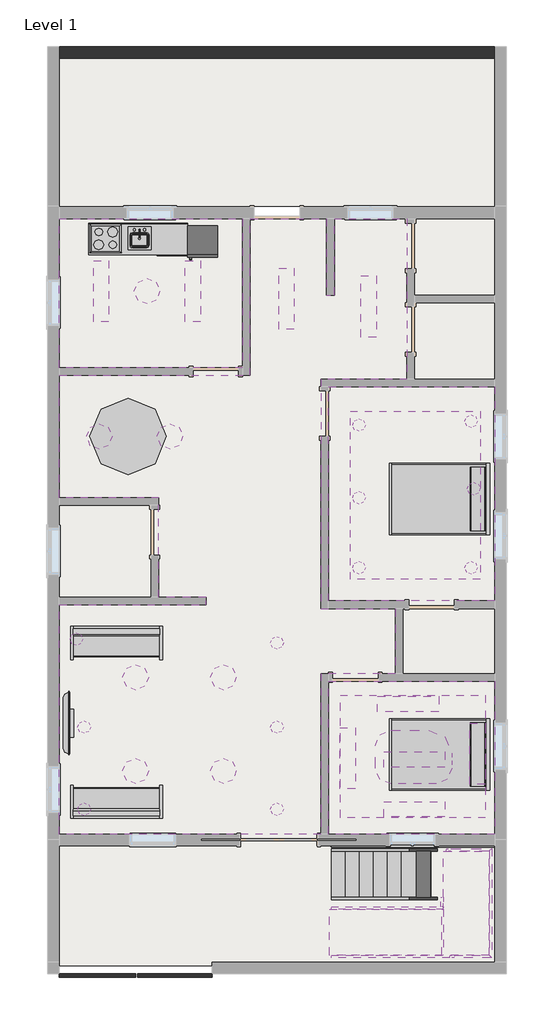
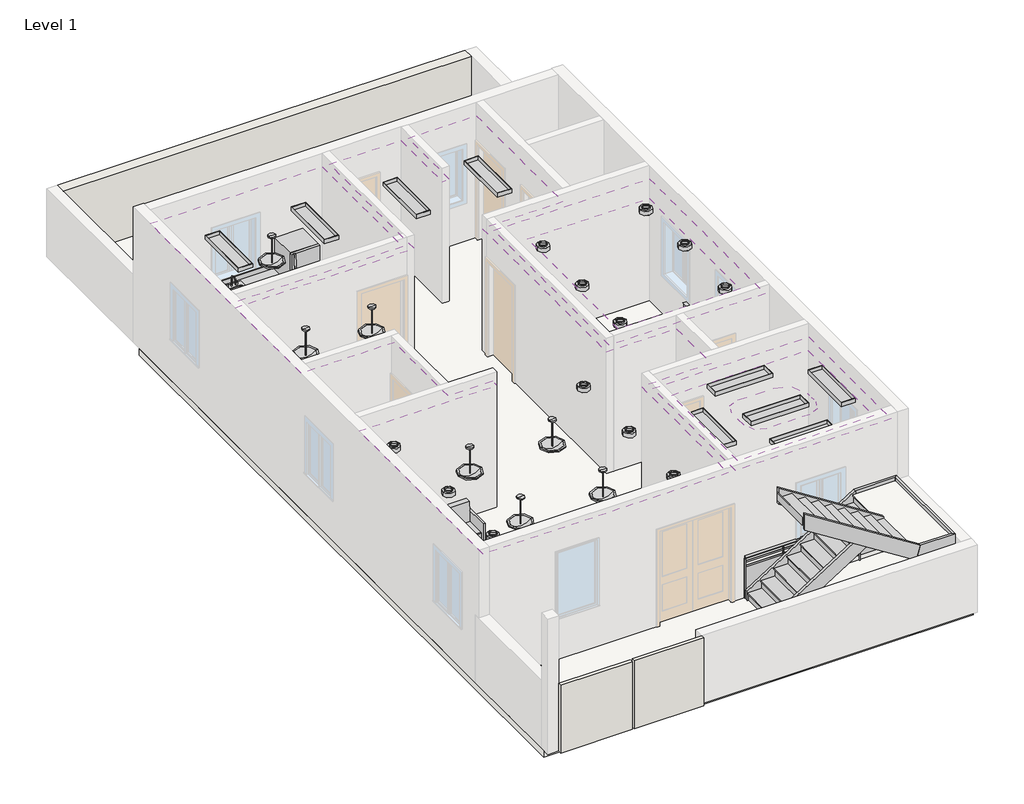
# One storey, part 2 of 2: 28 light fixtures, 8 members, 7 coverings, 7 furniture elements, 4 proxies, 3 slabs, 2 stair flights, 2 walls, 2 other elements.
"""IFC4 building model written with IfcOpenShell, lengths in millimetres."""

from ifc_helpers import new_model, si_unit, point, frame, frame_2d, origin, origin_with_axes, place, context, project, spatial, polyline, circle_curve, ellipse_curve, trimmed, segment, composite_curve, outline, extrude, faceted_brep, transform, mapped, element, save
from ifc_brep_helpers import plane_surface, extruded_surface, advanced_brep
from components import proxy_a6faaae8, proxy_45b28599, kitchenette_medium_kitchenette_medium_844211aa, proxy_c523a7b7, flow_terminal_871c2e40, furniture_096e7f55, furniture_c6510c7c, m_sofa_1830mm_f9e8a66b, furniture_fdf74506, furniture_bbcc68ce, ceiling_light_flat_round_60w_120v_0a96185f, ceiling_light_linear_box_1_x4_1_lamp_120v_8873ebfc, pendant_light_hemisphere_100w_120v_9c66a66f, non_monolithic_landing_9c4d403a, stair_flight_350f2e97, stair_flight_9d7122d5, walls_1_walls_1_5f19503e

model = new_model("IFC4")

# Units and contexts
model_context = context("Model", 3, world=origin())
ifc_project = project(units=[si_unit("LENGTHUNIT", "METRE", prefix="MILLI")], contexts=[model_context])

# Site, building, storey
site = spatial("IfcSite", under=ifc_project)
building = spatial("IfcBuilding", under=site)
storey = spatial("IfcBuildingStorey", under=building, Name="Level 1", Elevation=0.0)

# Proxies
placement = place(None, origin())
proxy_shape = proxy_a6faaae8(model_context)
element("IfcBuildingElementProxy", 1, Name="Cook Top-4 Unit2 : 22\" x 20\"", ObjectType="Cook Top-4 Unit2 : 22\" x 20\"", at=placement, inside=storey, context=model_context, shape_type="MappedRepresentation", body=[
    mapped(proxy_shape, transform((-8913.4692849, 13575.3206867, 0.0), x_axis=(1.0, 0.0, 0.0), y_axis=(0.0, 1.0, 0.0), z_axis=(0.0, 0.0, 1.0))),
])
proxy_2_shape = proxy_45b28599(model_context)
element("IfcBuildingElementProxy", 2, Name="Dishwasher : 24\" x 24\" x 34\"", ObjectType="Dishwasher : 24\" x 24\" x 34\"", at=placement, inside=storey, context=model_context, shape_type="MappedRepresentation", body=[
    mapped(proxy_2_shape, transform((-7962.2867534, 13283.4711219, 0.0), x_axis=(1.0, 0.0, 0.0), y_axis=(0.0, 1.0, 0.0), z_axis=(0.0, 0.0, 1.0))),
])
kitchenette_medium_kitchenette_medium_shape = kitchenette_medium_kitchenette_medium_844211aa(model_context)
element("IfcBuildingElementProxy", 3, Name="Kitchenette - Medium : Kitchenette - Medium", ObjectType="Kitchenette - Medium : Kitchenette - Medium", at=placement, inside=storey, context=model_context, shape_type="MappedRepresentation", body=[
    mapped(kitchenette_medium_kitchenette_medium_shape, transform((-8589.3069898, 13880.1206867, 0.0), x_axis=(1.0, 0.0, 0.0), y_axis=(0.0, 1.0, 0.0), z_axis=(0.0, 0.0, 1.0))),
])
proxy_3_shape = proxy_c523a7b7(model_context)
element("IfcBuildingElementProxy", 4, Name="Refrigerator : 24\" x 25\" LH", ObjectType="Refrigerator : 24\" x 25\" LH", at=placement, inside=storey, context=model_context, shape_type="MappedRepresentation", body=[
    mapped(proxy_3_shape, transform((-6976.7192849, 13529.6717152, 0.0), x_axis=(1.0, 0.0, 0.0), y_axis=(0.0, 1.0, 0.0), z_axis=(0.0, 0.0, 1.0))),
])

# Coverings
element("IfcCovering", 5, ObjectType="2' x 4' ACT System", at=placement, inside=storey, context=model_context, shape_type="SweptSolid", body=[
    extrude(outline(polyline([(-1153.7692849, 6349.0206867), (-4468.4692849, 6349.0206867), (-4468.4692849, 10616.2206867), (-1153.7692849, 10616.2206867), (-1153.7692849, 6349.0206867)])), frame((0.0, 0.0, 2743.2), z_axis=(0.0, 0.0, 1.0), x_axis=(1.0, 0.0, 0.0)), (0.0, 0.0, 1.0), 57.15),
])
element("IfcCovering", 6, ObjectType="2' x 4' ACT System", at=placement, inside=storey, context=model_context, shape_type="SweptSolid", body=[
    extrude(outline(polyline([(-1153.7692849, 1700.8206867), (-4468.4692849, 1700.8206867), (-4468.4692849, 4748.8206867), (-1153.7692849, 4748.8206867), (-1153.7692849, 1700.8206867)])), frame((0.0, 0.0, 2743.2), z_axis=(0.0, 0.0, 1.0), x_axis=(1.0, 0.0, 0.0)), (0.0, 0.0, 1.0), 57.15),
])
element("IfcCovering", 7, ObjectType="2' x 4' ACT System", at=placement, inside=storey, context=model_context, shape_type="SweptSolid", body=[
    extrude(outline(polyline([(-4620.8692849, 4901.2206867), (-4620.8692849, 1700.8206867), (-9840.5692849, 1700.8206867), (-9840.5692849, 6272.8206867), (-6906.8692849, 6272.8206867), (-6906.8692849, 6425.2206867), (-7859.3692849, 6425.2206867), (-7859.3692849, 8406.4206867), (-9840.5692849, 8406.4206867), (-9840.5692849, 10844.8206867), (-6030.5692849, 10844.8206867), (-6030.5692849, 13969.0206867), (-4506.5692849, 13969.0206867), (-4506.5692849, 12445.0206867), (-4354.1692849, 12445.0206867), (-4354.1692849, 13969.0206867), (-2906.3692849, 13969.0206867), (-2906.3692849, 10768.6206867), (-4620.8692849, 10768.6206867), (-4620.8692849, 6196.6206867), (-3134.9692849, 6196.6206867), (-3134.9692849, 4901.2206867), (-4620.8692849, 4901.2206867)])), frame((0.0, 0.0, 2743.2), z_axis=(0.0, 0.0, 1.0), x_axis=(1.0, 0.0, 0.0)), (0.0, 0.0, 1.0), 57.15),
])
element("IfcCovering", 8, ObjectType="2' x 4' ACT System", at=placement, inside=storey, context=model_context, shape_type="SweptSolid", body=[
    extrude(outline(polyline([(-9840.5692849, 13969.0206867), (-6182.9692849, 13969.0206867), (-6182.9692849, 10997.2206867), (-9840.5692849, 10997.2206867), (-9840.5692849, 13969.0206867)])), frame((0.0, 0.0, 2743.2), z_axis=(0.0, 0.0, 1.0), x_axis=(1.0, 0.0, 0.0)), (0.0, 0.0, 1.0), 57.15),
])
element("IfcCovering", 9, ObjectType="design", at=placement, inside=storey, context=model_context, shape_type="SweptSolid", body=[
    extrude(outline(polyline([(-1440.6811411, 10131.5450067), (-1440.6811411, 6778.7450067), (-4031.4811411, 6778.7450067), (-4031.4811411, 10131.5450067), (-1440.6811411, 10131.5450067)]), holes=[composite_curve([segment(polyline([(-1960.6193665, 9832.8150154), (-3523.4811411, 9832.8150154)]), True, "CONTINUOUS"), segment(trimmed(circle_curve(frame_2d((-3523.4811411, 9629.6150154)), 203.2), [point((-3523.4811411, 9832.8150154))], [point((-3726.6811411, 9629.6150154))], True, "CARTESIAN"), True, "CONTINUOUS"), segment(polyline([(-3726.6811411, 9629.6150154), (-3726.6811411, 7369.0150154)]), True, "CONTINUOUS"), segment(trimmed(circle_curve(frame_2d((-3396.4811411, 7369.0150154)), 330.2), [point((-3726.6811411, 7369.0150154))], [point((-3396.4811411, 7038.8150154))], True, "CARTESIAN"), True, "CONTINUOUS"), segment(polyline([(-3396.4811411, 7038.8150154), (-2177.2811411, 7038.8150154)]), True, "CONTINUOUS"), segment(trimmed(circle_curve(frame_2d((-2177.2811411, 7470.6150154)), 431.8), [point((-2177.2811411, 7038.8150154))], [point((-1745.4811411, 7470.6150154))], True, "CARTESIAN"), True, "CONTINUOUS"), segment(polyline([(-1745.4811411, 7470.6150154), (-1745.4811411, 9617.67679)]), True, "CONTINUOUS"), segment(trimmed(circle_curve(frame_2d((-1960.6193665, 9617.67679)), 215.1382254), [point((-1745.4811411, 9617.67679))], [point((-1960.6193665, 9832.8150154))], True, "CARTESIAN"), True, "CONTINUOUS")], self_intersect=False)]), frame((0.0, 0.0, 2692.4), z_axis=(0.0, 0.0, 1.0), x_axis=(1.0, 0.0, 0.0)), (0.0, 0.0, 1.0), 50.8),
])
element("IfcCovering", 10, ObjectType="design", at=placement, inside=storey, context=model_context, shape_type="SweptSolid", body=[
    extrude(outline(polyline([(-1336.3091854, 4467.6615302), (-1336.3091854, 2029.2615302), (-4231.9091854, 2029.2615302), (-4231.9091854, 4467.6615302), (-1336.3091854, 4467.6615302)]), holes=[polyline([(-1663.6359703, 4145.0635701), (-3949.6359703, 4145.0635701), (-3949.6359703, 2316.2635701), (-1663.6359703, 2316.2635701), (-1663.6359703, 4145.0635701)])]), frame((0.0, 0.0, 2679.6205268), z_axis=(0.0, 0.0, 1.0), x_axis=(1.0, 0.0, 0.0)), (0.0, 0.0, 1.0), 50.8),
])
element("IfcCovering", 11, ObjectType="inner", at=placement, inside=storey, context=model_context, shape_type="SweptSolid", body=[
    extrude(outline(composite_curve([segment(trimmed(circle_curve(frame_2d((-2466.1469386, 3312.9178401)), 457.2), [point((-2466.1469386, 3770.1178401))], [point((-2008.9469386, 3312.9178401))], False, "CARTESIAN"), True, "CONTINUOUS"), segment(polyline([(-2008.9469386, 3312.9178401), (-2008.9469386, 3008.1178401)]), True, "CONTINUOUS"), segment(trimmed(circle_curve(frame_2d((-2313.7469386, 3008.1178401)), 304.8), [point((-2008.9469386, 3008.1178401))], [point((-2313.7469386, 2703.3178401))], False, "CARTESIAN"), True, "CONTINUOUS"), segment(polyline([(-2313.7469386, 2703.3178401), (-3228.1469386, 2703.3178401)]), True, "CONTINUOUS"), segment(trimmed(circle_curve(frame_2d((-3228.1469386, 3008.1178401)), 304.8), [point((-3228.1469386, 2703.3178401))], [point((-3532.9469386, 3008.1178401))], False, "CARTESIAN"), True, "CONTINUOUS"), segment(polyline([(-3532.9469386, 3008.1178401), (-3532.9469386, 3465.3178401)]), True, "CONTINUOUS"), segment(trimmed(circle_curve(frame_2d((-3228.1469386, 3465.3178401)), 304.8), [point((-3532.9469386, 3465.3178401))], [point((-3228.1469386, 3770.1178401))], False, "CARTESIAN"), True, "CONTINUOUS"), segment(polyline([(-3228.1469386, 3770.1178401), (-2466.1469386, 3770.1178401)]), True, "CONTINUOUS")], self_intersect=False)), frame((0.0, 0.0, 2641.6), z_axis=(0.0, 0.0, 1.0), x_axis=(1.0, 0.0, 0.0)), (0.0, 0.0, 1.0), 50.8),
])

# Flow terminal
flow_terminal_shape = flow_terminal_871c2e40(model_context)
element("IfcFlowTerminal", 12, ObjectType="Sink Kitchen-Island : 18\" x 18\"", at=placement, inside=storey, context=model_context, shape_type="MappedRepresentation", body=[
    mapped(flow_terminal_shape, transform((-8256.0585254, 13572.9752855, -14.4), x_axis=(1.0, 0.0, 0.0), y_axis=(0.0, 1.0, 0.0), z_axis=(0.0, 0.0, 1.0))),
])

# Furniture
furniture_shape = furniture_096e7f55(model_context)
element("IfcFurniture", 13, ObjectType="Bed-Shaker : Double 56\" x 78\"", at=placement, inside=storey, context=model_context, shape_type="MappedRepresentation", body=[
    mapped(furniture_shape, transform((-1268.0692849, 8361.9706867, 0.0), x_axis=(0.0, -1.0000000000000007, 0.0), y_axis=(1.0000000000000007, 0.0, 0.0), z_axis=(0.0, 0.0, 1.0))),
])
element("IfcFurniture", 14, ObjectType="Bed-Shaker : Double 56\" x 78\"", at=placement, inside=storey, context=model_context, shape_type="MappedRepresentation", body=[
    mapped(furniture_shape, transform((-1268.0692849, 3269.2706867, 0.0), x_axis=(0.0, -1.0, 0.0), y_axis=(1.0, 0.0, 0.0), z_axis=(0.0, 0.0, 1.0))),
])
furniture_2_shape = furniture_c6510c7c(model_context)
element("IfcFurniture", 15, ObjectType="Counter Top w Sink Hole : 24\" Depth", at=placement, inside=storey, context=model_context, shape_type="MappedRepresentation", body=[
    mapped(furniture_2_shape, transform((-8055.9069898, 13880.1206867, -14.4), x_axis=(1.0, 0.0, 0.0), y_axis=(0.0, 1.0, 0.0), z_axis=(0.0, 0.0, 1.0))),
])
m_sofa_1830mm_shape = m_sofa_1830mm_f9e8a66b(model_context)
element("IfcFurniture", 16, ObjectType="M_Sofa : 1830mm", at=placement, inside=storey, context=model_context, shape_type="MappedRepresentation", body=[
    mapped(m_sofa_1830mm_shape, transform((-8767.9397767, 5364.6665883, 0.0), x_axis=(1.0, 0.0, 0.0), y_axis=(0.0, 1.0, 0.0), z_axis=(0.0, 0.0, 1.0))),
])
element("IfcFurniture", 17, ObjectType="M_Sofa : 1830mm", at=placement, inside=storey, context=model_context, shape_type="MappedRepresentation", body=[
    mapped(m_sofa_1830mm_shape, transform((-8627.1987931, 2494.674785, 0.0), x_axis=(-1.0000000000000002, 0.0, 0.0), y_axis=(0.0, -1.0000000000000002, 0.0), z_axis=(0.0, 0.0, 1.0))),
])
furniture_3_shape = furniture_fdf74506(model_context)
element("IfcFurniture", 18, ObjectType="TV - Flat Screen : 50\"", at=placement, inside=storey, context=model_context, shape_type="MappedRepresentation", body=[
    mapped(furniture_3_shape, transform((-9706.3630954, 3915.2652008, 0.0), x_axis=(0.0, 1.0000000000000007, 0.0), y_axis=(-1.0000000000000007, 0.0, 0.0), z_axis=(0.0, 0.0, 1.0))),
])
furniture_4_shape = furniture_bbcc68ce(model_context)
element("IfcFurniture", 19, ObjectType="Table-Dining Round w Chairs : 60\" Diameter", at=placement, inside=storey, context=model_context, shape_type="MappedRepresentation", body=[
    mapped(furniture_4_shape, transform((-8572.6512521, 9810.4993752, 0.0), x_axis=(1.0, 0.0, 0.0), y_axis=(0.0, 1.0, 0.0), z_axis=(0.0, 0.0, 1.0))),
])

# Light fixtures
ceiling_light_flat_round_60w_120v_shape = ceiling_light_flat_round_60w_120v_0a96185f(model_context)
element("IfcLightFixture", 20, ObjectType="Ceiling Light - Flat Round : 60W - 120V", at=placement, inside=storey, context=model_context, shape_type="MappedRepresentation", body=[
    mapped(ceiling_light_flat_round_60w_120v_shape, transform((-9497.6692849, 5587.0206867, 304.8), x_axis=(1.0, 0.0, 0.0), y_axis=(0.0, 1.0, 0.0), z_axis=(0.0, 0.0, 1.0))),
])
element("IfcLightFixture", 21, ObjectType="Ceiling Light - Flat Round : 60W - 120V", at=placement, inside=storey, context=model_context, shape_type="MappedRepresentation", body=[
    mapped(ceiling_light_flat_round_60w_120v_shape, transform((-5497.1692849, 5510.8206867, 304.8), x_axis=(1.0, 0.0, 0.0), y_axis=(0.0, 1.0, 0.0), z_axis=(0.0, 0.0, 1.0))),
])
element("IfcLightFixture", 22, ObjectType="Ceiling Light - Flat Round : 60W - 120V", at=placement, inside=storey, context=model_context, shape_type="MappedRepresentation", body=[
    mapped(ceiling_light_flat_round_60w_120v_shape, transform((-9345.2692849, 3834.4206867, 304.8), x_axis=(1.0, 0.0, 0.0), y_axis=(0.0, 1.0, 0.0), z_axis=(0.0, 0.0, 1.0))),
])
element("IfcLightFixture", 23, ObjectType="Ceiling Light - Flat Round : 60W - 120V", at=placement, inside=storey, context=model_context, shape_type="MappedRepresentation", body=[
    mapped(ceiling_light_flat_round_60w_120v_shape, transform((-5497.1692849, 3834.4206867, 304.8), x_axis=(1.0, 0.0, 0.0), y_axis=(0.0, 1.0, 0.0), z_axis=(0.0, 0.0, 1.0))),
])
element("IfcLightFixture", 24, ObjectType="Ceiling Light - Flat Round : 60W - 120V", at=placement, inside=storey, context=model_context, shape_type="MappedRepresentation", body=[
    mapped(ceiling_light_flat_round_60w_120v_shape, transform((-9345.2692849, 2196.1206867, 304.8), x_axis=(1.0, 0.0, 0.0), y_axis=(0.0, 1.0, 0.0), z_axis=(0.0, 0.0, 1.0))),
])
element("IfcLightFixture", 25, ObjectType="Ceiling Light - Flat Round : 60W - 120V", at=placement, inside=storey, context=model_context, shape_type="MappedRepresentation", body=[
    mapped(ceiling_light_flat_round_60w_120v_shape, transform((-5497.1692849, 2196.1206867, 304.8), x_axis=(1.0, 0.0, 0.0), y_axis=(0.0, 1.0, 0.0), z_axis=(0.0, 0.0, 1.0))),
])
element("IfcLightFixture", 26, ObjectType="Ceiling Light - Flat Round : 60W - 277V", at=placement, inside=storey, context=model_context, shape_type="MappedRepresentation", body=[
    mapped(ceiling_light_flat_round_60w_120v_shape, transform((-3858.8692849, 9854.2206867, 254.0), x_axis=(1.0, 0.0, 0.0), y_axis=(0.0, 1.0, 0.0), z_axis=(0.0, 0.0, 1.0))),
])
element("IfcLightFixture", 27, ObjectType="Ceiling Light - Flat Round : 60W - 277V", at=placement, inside=storey, context=model_context, shape_type="MappedRepresentation", body=[
    mapped(ceiling_light_flat_round_60w_120v_shape, transform((-1623.6692849, 9930.4206867, 254.0), x_axis=(1.0, 0.0, 0.0), y_axis=(0.0, 1.0, 0.0), z_axis=(0.0, 0.0, 1.0))),
])
element("IfcLightFixture", 28, ObjectType="Ceiling Light - Flat Round : 60W - 277V", at=placement, inside=storey, context=model_context, shape_type="MappedRepresentation", body=[
    mapped(ceiling_light_flat_round_60w_120v_shape, transform((-1572.8692849, 8584.2206867, 254.0), x_axis=(1.0, 0.0, 0.0), y_axis=(0.0, 1.0, 0.0), z_axis=(0.0, 0.0, 1.0))),
])
element("IfcLightFixture", 29, ObjectType="Ceiling Light - Flat Round : 60W - 277V", at=placement, inside=storey, context=model_context, shape_type="MappedRepresentation", body=[
    mapped(ceiling_light_flat_round_60w_120v_shape, transform((-3858.8692849, 8406.4206867, 254.0), x_axis=(1.0, 0.0, 0.0), y_axis=(0.0, 1.0, 0.0), z_axis=(0.0, 0.0, 1.0))),
])
element("IfcLightFixture", 30, ObjectType="Ceiling Light - Flat Round : 60W - 277V", at=placement, inside=storey, context=model_context, shape_type="MappedRepresentation", body=[
    mapped(ceiling_light_flat_round_60w_120v_shape, transform((-3858.8692849, 7009.4206867, 254.0), x_axis=(1.0, 0.0, 0.0), y_axis=(0.0, 1.0, 0.0), z_axis=(0.0, 0.0, 1.0))),
])
element("IfcLightFixture", 31, ObjectType="Ceiling Light - Flat Round : 60W - 277V", at=placement, inside=storey, context=model_context, shape_type="MappedRepresentation", body=[
    mapped(ceiling_light_flat_round_60w_120v_shape, transform((-1623.6692849, 7009.4206867, 254.0), x_axis=(1.0, 0.0, 0.0), y_axis=(0.0, 1.0, 0.0), z_axis=(0.0, 0.0, 1.0))),
])
ceiling_light_linear_box_1_x4_1_lamp_120v_shape = ceiling_light_linear_box_1_x4_1_lamp_120v_8873ebfc(model_context)
element("IfcLightFixture", 32, ObjectType="Ceiling Light - Linear Box : 1'x4'(1 Lamp) - 120V", at=placement, inside=storey, context=model_context, shape_type="MappedRepresentation", body=[
    mapped(ceiling_light_linear_box_1_x4_1_lamp_120v_shape, transform((-9002.3692849, 12521.2206867, 304.8), x_axis=(0.0, 1.0000000000000002, 0.0), y_axis=(-1.0000000000000002, 0.0, 0.0), z_axis=(0.0, 0.0, 1.0))),
])
element("IfcLightFixture", 33, ObjectType="Ceiling Light - Linear Box : 1'x4'(1 Lamp) - 120V", at=placement, inside=storey, context=model_context, shape_type="MappedRepresentation", body=[
    mapped(ceiling_light_linear_box_1_x4_1_lamp_120v_shape, transform((-7173.5692849, 12521.2206867, 304.8), x_axis=(0.0, -1.0000000000000007, 0.0), y_axis=(1.0000000000000007, 0.0, 0.0), z_axis=(0.0, 0.0, 1.0))),
])
element("IfcLightFixture", 34, ObjectType="Ceiling Light - Linear Box : 1'x4'(1 Lamp) - 120V", at=placement, inside=storey, context=model_context, shape_type="MappedRepresentation", body=[
    mapped(ceiling_light_linear_box_1_x4_1_lamp_120v_shape, transform((-3668.3692849, 12216.4206867, 304.8), x_axis=(0.0, 1.0000000000000002, 0.0), y_axis=(-1.0000000000000002, 0.0, 0.0), z_axis=(0.0, 0.0, 1.0))),
])
element("IfcLightFixture", 35, ObjectType="Ceiling Light - Linear Box : 1'x4'(1 Lamp) - 120V", at=placement, inside=storey, context=model_context, shape_type="MappedRepresentation", body=[
    mapped(ceiling_light_linear_box_1_x4_1_lamp_120v_shape, transform((-5306.6692849, 12368.8206867, 304.8), x_axis=(0.0, 1.0000000000000002, 0.0), y_axis=(-1.0000000000000002, 0.0, 0.0), z_axis=(0.0, 0.0, 1.0))),
])
element("IfcLightFixture", 36, ObjectType="Ceiling Light - Linear Box : 1'x4'(2 Lamp) - 120V", at=placement, inside=storey, context=model_context, shape_type="MappedRepresentation", body=[
    mapped(ceiling_light_linear_box_1_x4_1_lamp_120v_shape, transform((-2753.9692849, 3186.7206867, 203.2), x_axis=(1.0, 0.0, 0.0), y_axis=(0.0, 1.0, 0.0), z_axis=(0.0, 0.0, 1.0))),
])
element("IfcLightFixture", 37, ObjectType="Ceiling Light - Linear Box : 1'x4'(2 Lamp) - 120V", at=placement, inside=storey, context=model_context, shape_type="MappedRepresentation", body=[
    mapped(ceiling_light_linear_box_1_x4_1_lamp_120v_shape, transform((-2880.9692849, 4291.6206867, 241.2205268), x_axis=(1.0, 0.0, 0.0), y_axis=(0.0, 1.0, 0.0), z_axis=(0.0, 0.0, 1.0))),
])
element("IfcLightFixture", 38, ObjectType="Ceiling Light - Linear Box : 1'x4'(2 Lamp) - 120V", at=placement, inside=storey, context=model_context, shape_type="MappedRepresentation", body=[
    mapped(ceiling_light_linear_box_1_x4_1_lamp_120v_shape, transform((-2753.9692849, 2196.1206867, 241.2205268), x_axis=(1.0, 0.0, 0.0), y_axis=(0.0, 1.0, 0.0), z_axis=(0.0, 0.0, 1.0))),
])
element("IfcLightFixture", 39, ObjectType="Ceiling Light - Linear Box : 1'x4'(2 Lamp) - 120V", at=placement, inside=storey, context=model_context, shape_type="MappedRepresentation", body=[
    mapped(ceiling_light_linear_box_1_x4_1_lamp_120v_shape, transform((-1496.6692849, 3301.0206867, 241.2205268), x_axis=(0.0, 1.0000000000000002, 0.0), y_axis=(-1.0000000000000002, 0.0, 0.0), z_axis=(0.0, 0.0, 1.0))),
])
element("IfcLightFixture", 40, ObjectType="Ceiling Light - Linear Box : 1'x4'(2 Lamp) - 120V", at=placement, inside=storey, context=model_context, shape_type="MappedRepresentation", body=[
    mapped(ceiling_light_linear_box_1_x4_1_lamp_120v_shape, transform((-4087.4692849, 3212.1206867, 241.2205268), x_axis=(0.0, 1.0000000000000002, 0.0), y_axis=(-1.0000000000000002, 0.0, 0.0), z_axis=(0.0, 0.0, 1.0))),
])
pendant_light_hemisphere_100w_120v_shape = pendant_light_hemisphere_100w_120v_9c66a66f(model_context)
element("IfcLightFixture", 41, ObjectType="Pendant Light - Hemisphere : 100W - 120V", at=placement, inside=storey, context=model_context, shape_type="MappedRepresentation", body=[
    mapped(pendant_light_hemisphere_100w_120v_shape, transform((-9040.4692849, 9625.6206867, 304.8), x_axis=(1.0, 0.0, 0.0), y_axis=(0.0, 1.0, 0.0), z_axis=(0.0, 0.0, 1.0))),
])
element("IfcLightFixture", 42, ObjectType="Pendant Light - Hemisphere : 100W - 120V", at=placement, inside=storey, context=model_context, shape_type="MappedRepresentation", body=[
    mapped(pendant_light_hemisphere_100w_120v_shape, transform((-7630.7692849, 9625.6206867, 304.8), x_axis=(1.0, 0.0, 0.0), y_axis=(0.0, 1.0, 0.0), z_axis=(0.0, 0.0, 1.0))),
])
element("IfcLightFixture", 43, ObjectType="Pendant Light - Hemisphere : 100W - 120V", at=placement, inside=storey, context=model_context, shape_type="MappedRepresentation", body=[
    mapped(pendant_light_hemisphere_100w_120v_shape, transform((-8087.9692849, 12521.2206867, 304.8), x_axis=(1.0, 0.0, 0.0), y_axis=(0.0, 1.0, 0.0), z_axis=(0.0, 0.0, 1.0))),
])
element("IfcLightFixture", 44, ObjectType="Pendant Light - Hemisphere : 100W - 120V", at=placement, inside=storey, context=model_context, shape_type="MappedRepresentation", body=[
    mapped(pendant_light_hemisphere_100w_120v_shape, transform((-8316.5692849, 2958.1206867, 304.8), x_axis=(1.0, 0.0, 0.0), y_axis=(0.0, 1.0, 0.0), z_axis=(0.0, 0.0, 1.0))),
])
element("IfcLightFixture", 45, ObjectType="Pendant Light - Hemisphere : 100W - 120V", at=placement, inside=storey, context=model_context, shape_type="MappedRepresentation", body=[
    mapped(pendant_light_hemisphere_100w_120v_shape, transform((-8316.5692849, 4825.0206867, 304.8), x_axis=(1.0, 0.0, 0.0), y_axis=(0.0, 1.0, 0.0), z_axis=(0.0, 0.0, 1.0))),
])
element("IfcLightFixture", 46, ObjectType="Pendant Light - Hemisphere : 100W - 120V", at=placement, inside=storey, context=model_context, shape_type="MappedRepresentation", body=[
    mapped(pendant_light_hemisphere_100w_120v_shape, transform((-6563.9692849, 4825.0206867, 304.8), x_axis=(1.0, 0.0, 0.0), y_axis=(0.0, 1.0, 0.0), z_axis=(0.0, 0.0, 1.0))),
])
element("IfcLightFixture", 47, ObjectType="Pendant Light - Hemisphere : 100W - 120V", at=placement, inside=storey, context=model_context, shape_type="MappedRepresentation", body=[
    mapped(pendant_light_hemisphere_100w_120v_shape, transform((-6563.9692849, 2958.1206867, 304.8), x_axis=(1.0, 0.0, 0.0), y_axis=(0.0, 1.0, 0.0), z_axis=(0.0, 0.0, 1.0))),
])

# Members
element("IfcMember", 48, ObjectType="Stringer - 2\" Width", at=placement, inside=storey, context=model_context, shape_type="SweptSolid", body=[
    extrude(outline(polyline([(215.0106437, -4413.813859), (0.0, -4413.813859), (0.0, -4183.9583297), (1371.6, -2028.5869011), (1676.4, -2117.3448705), (215.0106437, -4413.813859)])), frame((0.0, 1358.5428136, 0.0), z_axis=(0.0, 1.0, 0.0), x_axis=(0.0, 0.0, 1.0)), (0.0, 0.0, 1.0), 50.8),
])
element("IfcMember", 49, ObjectType="Stringer - 2\" Width", at=placement, inside=storey, context=model_context, shape_type="SweptSolid", body=[
    extrude(outline(polyline([(215.0106437, -4413.813859), (0.0, -4413.813859), (0.0, -4183.9583297), (1243.8010268, -2229.413859), (1605.083371, -2229.413859), (215.0106437, -4413.813859)])), frame((0.0, 393.3428136, 0.0), z_axis=(0.0, 1.0, 0.0), x_axis=(0.0, 0.0, 1.0)), (0.0, 0.0, 1.0), 50.8),
])
element("IfcMember", 50, ObjectType="Stringer - 2\" Width", at=placement, inside=storey, context=model_context, shape_type="SweptSolid", body=[
    extrude(outline(polyline([(1371.6, -2049.2408169), (1676.4, -1960.4828475), (3237.6106437, -4413.813859), (2876.3282995, -4413.813859), (1371.6, -2049.2408169)])), frame((0.0, -762.9793133, 0.0), z_axis=(0.0, 1.0, 0.0), x_axis=(0.0, 0.0, 1.0)), (0.0, 0.0, 1.0), 50.8),
])
element("IfcMember", 51, ObjectType="Stringer - 2\" Width", at=placement, inside=storey, context=model_context, shape_type="SweptSolid", body=[
    extrude(outline(polyline([(1453.9282995, -2178.613859), (1815.2106437, -2178.613859), (3237.6106437, -4413.813859), (2876.3282995, -4413.813859), (1453.9282995, -2178.613859)])), frame((0.0, 202.2206867, 0.0), z_axis=(0.0, 1.0, 0.0), x_axis=(0.0, 0.0, 1.0)), (0.0, 0.0, 1.0), 50.8),
])
element("IfcMember", 52, ObjectType="Stringer - 2\" Width", at=placement, inside=storey, context=model_context, shape_type="Brep", body=[
    faceted_brep([(-1960.4828475, -712.1793133, 1676.4), (-1960.4828475, -762.9793133, 1676.4), (-1213.413859, -762.9793133, 1676.4), (-1264.213859, -712.1793133, 1676.4), (-2049.2408169, -712.1793133, 1371.6), (-1264.213859, -712.1793133, 1371.6), (-2049.2408169, -762.9793133, 1371.6), (-1213.413859, -762.9793133, 1371.6)], [[[0, 1, 2, 3]], [[4, 0, 3, 5]], [[6, 4, 5, 7]], [[1, 6, 7, 2]], [[1, 0, 4, 6]], [[2, 7, 5, 3]]]),
])
element("IfcMember", 53, ObjectType="Stringer - 2\" Width", at=placement, inside=storey, context=model_context, shape_type="SweptSolid", body=[
    extrude(outline(polyline([(-1213.413859, -762.9793133), (-1264.213859, -712.1793133), (-1264.213859, 1358.5428136), (-1213.413859, 1409.3428136), (-1213.413859, -762.9793133)])), frame((0.0, 0.0, 1371.6), z_axis=(0.0, 0.0, 1.0), x_axis=(1.0, 0.0, 0.0)), (0.0, 0.0, 1.0), 304.8),
])
element("IfcMember", 54, ObjectType="Stringer - 2\" Width", at=placement, inside=storey, context=model_context, shape_type="Brep", body=[
    faceted_brep([(-1264.213859, 1358.5428136, 1676.4), (-1213.413859, 1409.3428136, 1676.4), (-2117.3448705, 1409.3428136, 1676.4), (-2117.3448705, 1358.5428136, 1676.4), (-1264.213859, 1358.5428136, 1371.6), (-2028.5869011, 1358.5428136, 1371.6), (-1213.413859, 1409.3428136, 1371.6), (-2028.5869011, 1409.3428136, 1371.6)], [[[0, 1, 2, 3]], [[4, 0, 3, 5]], [[6, 4, 5, 7]], [[1, 6, 7, 2]], [[1, 0, 4, 6]], [[2, 7, 5, 3]]]),
])
element("IfcMember", 55, ObjectType="Stringer - 2\" Width", at=placement, inside=storey, context=model_context, shape_type="SweptSolid", body=[
    extrude(outline(polyline([(-2229.413859, 444.1428136), (-2178.613859, 444.1428136), (-2178.613859, 253.0206867), (-2229.413859, 253.0206867), (-2229.413859, 444.1428136)])), frame((0.0, 0.0, 1371.6), z_axis=(0.0, 0.0, 1.0), x_axis=(1.0, 0.0, 0.0)), (0.0, 0.0, 1.0), 304.8),
])

# Railing
element("IfcRailing", 56, ObjectType="Glass Panel - Bottom Fill", at=placement, inside=storey, context=model_context, shape_type="SolidModel", body=[
    advanced_brep(
    [(-1153.7692849, 1434.1206867, 914.4), (-1153.7692849, 1510.3206867, 914.4), (-4412.1017807, 1434.1206867, 914.4), (-4412.1017807, 1510.3206867, 914.4)],
    [
        (0, 1, ellipse_curve(frame((-1153.7692849, 1472.2206867, 914.4), z_axis=(1.0, 0.0, 0.0), x_axis=(0.0, 1.0, 0.0)), 38.1, 28.575)),
        (1, 0, ellipse_curve(frame((-1153.7692849, 1472.2206867, 914.4), z_axis=(1.0, 0.0, 0.0), x_axis=(0.0, 1.0, 0.0)), 38.1, 28.575)),
        (2, 3, ellipse_curve(frame((-4412.1017807, 1472.2206867, 914.4), z_axis=(-1.0, 0.0, 0.0), x_axis=(0.0, 1.0, 0.0)), 38.1, 28.575)),
        (3, 2, ellipse_curve(frame((-4412.1017807, 1472.2206867, 914.4), z_axis=(-1.0, 0.0, 0.0), x_axis=(0.0, 1.0, 0.0)), 38.1, 28.575)),
        (0, 2),
        (3, 1),
    ],
    [
        plane_surface(frame((-1153.7692849, 1472.2206867, 914.4), z_axis=(1.0, 0.0, 0.0), x_axis=(0.0, -1.0, 0.0))),
        plane_surface(frame((-4412.1017807, 1472.2206867, 914.4), z_axis=(-1.0, 0.0, 0.0), x_axis=(0.0, -1.0, 0.0))),
        extruded_surface(trimmed(ellipse_curve(frame((-4412.1017807, 1472.2206867, 914.4), z_axis=(1.0, 0.0, 0.0), x_axis=(0.0, 1.0, 0.0)), 38.1, 28.575), [point((-4412.1017807, 1434.1206867, 914.4))], [point((-4412.1017807, 1510.3206867, 914.4))], True, "CARTESIAN"), (3258.3324958, 0.0, 0.0), 3258.3324958),
        extruded_surface(trimmed(ellipse_curve(frame((-4412.1017807, 1472.2206867, 914.4), z_axis=(1.0, 0.0, 0.0), x_axis=(0.0, 1.0, 0.0)), 38.1, 28.575), [point((-4412.1017807, 1510.3206867, 914.4))], [point((-4412.1017807, 1434.1206867, 914.4))], True, "CARTESIAN"), (3258.3324958, 0.0, 0.0), 3258.3324958),
    ],
    [
        (0, [[1, 2]]),
        (1, [[3, 4]]),
        (2, [[-1, 5, -4, 6]]),
        (3, [[-2, -6, -3, -5]]),
    ],
),
    extrude(outline(polyline([(-1153.7692849, 1484.9206867), (-1153.7692849, 1459.5206867), (-4412.1017807, 1459.5206867), (-4412.1017807, 1484.9206867), (-1153.7692849, 1484.9206867)])), frame((0.0, 0.0, 800.1), z_axis=(0.0, 0.0, 1.0), x_axis=(1.0, 0.0, 0.0)), (0.0, 0.0, 1.0), 25.4),
    extrude(outline(polyline([(-1153.7692849, 1484.9206867), (-1153.7692849, 1459.5206867), (-4412.1017807, 1459.5206867), (-4412.1017807, 1484.9206867), (-1153.7692849, 1484.9206867)])), frame((0.0, 0.0, 698.5), z_axis=(0.0, 0.0, 1.0), x_axis=(1.0, 0.0, 0.0)), (0.0, 0.0, 1.0), 25.4),
    extrude(outline(polyline([(-4402.1855328, 1497.6206867), (-4402.1855328, 1446.8206867), (-4414.8855328, 1446.8206867), (-4414.8855328, 1497.6206867), (-4402.1855328, 1497.6206867)])), origin_with_axes(), (0.0, 0.0, 1.0), 885.6788223),
    extrude(outline(polyline([(-3595.7355328, 1465.6855296), (-4408.5355328, 1465.6855296), (-4408.5355328, 1472.0355296), (-3595.7355328, 1472.0355296), (-3595.7355328, 1465.6855296)])), frame((0.0, 0.0, 101.6), z_axis=(0.0, 0.0, 1.0), x_axis=(1.0, 0.0, 0.0)), (0.0, 0.0, 1.0), 596.9),
    extrude(outline(polyline([(-3589.3855328, 1497.6206867), (-3589.3855328, 1446.8206867), (-3602.0855328, 1446.8206867), (-3602.0855328, 1497.6206867), (-3589.3855328, 1497.6206867)])), origin_with_axes(), (0.0, 0.0, 1.0), 885.6788223),
    extrude(outline(polyline([(-2782.9355328, 1465.6855296), (-3595.7355328, 1465.6855296), (-3595.7355328, 1472.0355296), (-2782.9355328, 1472.0355296), (-2782.9355328, 1465.6855296)])), frame((0.0, 0.0, 101.6), z_axis=(0.0, 0.0, 1.0), x_axis=(1.0, 0.0, 0.0)), (0.0, 0.0, 1.0), 596.9),
    extrude(outline(polyline([(-2776.5855328, 1497.6206867), (-2776.5855328, 1446.8206867), (-2789.2855328, 1446.8206867), (-2789.2855328, 1497.6206867), (-2776.5855328, 1497.6206867)])), origin_with_axes(), (0.0, 0.0, 1.0), 885.6788223),
    extrude(outline(polyline([(-1970.1355328, 1465.6855296), (-2782.9355328, 1465.6855296), (-2782.9355328, 1472.0355296), (-1970.1355328, 1472.0355296), (-1970.1355328, 1465.6855296)])), frame((0.0, 0.0, 101.6), z_axis=(0.0, 0.0, 1.0), x_axis=(1.0, 0.0, 0.0)), (0.0, 0.0, 1.0), 596.9),
    extrude(outline(polyline([(-1963.7855328, 1497.6206867), (-1963.7855328, 1446.8206867), (-1976.4855328, 1446.8206867), (-1976.4855328, 1497.6206867), (-1963.7855328, 1497.6206867)])), origin_with_axes(), (0.0, 0.0, 1.0), 885.6788223),
    extrude(outline(polyline([(-1157.3355328, 1465.6855296), (-1970.1355328, 1465.6855296), (-1970.1355328, 1472.0355296), (-1157.3355328, 1472.0355296), (-1157.3355328, 1465.6855296)])), frame((0.0, 0.0, 101.6), z_axis=(0.0, 0.0, 1.0), x_axis=(1.0, 0.0, 0.0)), (0.0, 0.0, 1.0), 596.9),
    extrude(outline(polyline([(-1150.9855328, 1497.6206867), (-1150.9855328, 1446.8206867), (-1163.6855328, 1446.8206867), (-1163.6855328, 1497.6206867), (-1150.9855328, 1497.6206867)])), origin_with_axes(), (0.0, 0.0, 1.0), 885.6788223),
    extrude(outline(polyline([(-4399.4017807, 1481.7456867), (-4399.4017807, 1462.6956867), (-4418.4517807, 1462.6956867), (-4418.4517807, 1481.7456867), (-4399.4017807, 1481.7456867)])), origin_with_axes(), (0.0, 0.0, 1.0), 885.6788223),
    extrude(outline(polyline([(-1147.4192849, 1481.7456867), (-1147.4192849, 1462.6956867), (-1166.4692849, 1462.6956867), (-1166.4692849, 1481.7456867), (-1147.4192849, 1481.7456867)])), origin_with_axes(), (0.0, 0.0, 1.0), 885.6788223),
])

# Slabs
element("IfcSlab", 57, ObjectType="6\"", at=placement, inside=storey, context=model_context, shape_type="SweptSolid", body=[
    extrude(outline(polyline([(-925.1692849, 13981.7206867), (-925.1692849, -928.0793133), (-10069.1692849, -928.0793133), (-10069.1692849, 13981.7206867), (-925.1692849, 13981.7206867)])), frame((0.0, 0.0, -152.4), z_axis=(0.0, 0.0, 1.0), x_axis=(1.0, 0.0, 0.0)), (0.0, 0.0, 1.0), 152.4),
])
non_monolithic_landing_shape = non_monolithic_landing_9c4d403a(model_context)
element("IfcSlab", 58, ObjectType="Non-Monolithic Landing", at=placement, inside=storey, context=model_context, shape_type="MappedRepresentation", body=[
    mapped(non_monolithic_landing_shape, transform((0.0, 0.0, 0.0), x_axis=(1.0, 0.0, 0.0), y_axis=(0.0, 1.0, 0.0), z_axis=(0.0, 0.0, 1.0))),
])
element("IfcSlab", 59, ObjectType="grass", at=placement, inside=storey, context=model_context, shape_type="SweptSolid", body=[
    extrude(outline(polyline([(-1153.7692849, 17169.4206867), (-1153.7692849, 14210.3206867), (-9840.5692849, 14210.3206867), (-9840.5692849, 17169.4206867), (-1153.7692849, 17169.4206867)])), frame((0.0, 0.0, -152.4), z_axis=(0.0, 0.0, 1.0), x_axis=(1.0, 0.0, 0.0)), (0.0, 0.0, 1.0), 152.4),
])

# Stair flights
stair_flight_shape = stair_flight_350f2e97(model_context)
element("IfcStairFlight", 60, ObjectType="2\" Tread 1\" Nosing 1/4\" Riser", at=placement, inside=storey, context=model_context, shape_type="MappedRepresentation", body=[
    mapped(stair_flight_shape, transform((0.0, 0.0, 0.0), x_axis=(1.0, 0.0, 0.0), y_axis=(0.0, 1.0, 0.0), z_axis=(0.0, 0.0, 1.0))),
])
stair_flight_2_shape = stair_flight_9d7122d5(model_context)
element("IfcStairFlight", 61, ObjectType="2\" Tread 1\" Nosing 1/4\" Riser", at=placement, inside=storey, context=model_context, shape_type="MappedRepresentation", body=[
    mapped(stair_flight_2_shape, transform((0.0, 0.0, 0.0), x_axis=(1.0, 0.0, 0.0), y_axis=(0.0, 1.0, 0.0), z_axis=(0.0, 0.0, 1.0))),
])

# Walls
element("IfcWall", 62, ObjectType="9\"", at=placement, inside=storey, context=model_context, shape_type="SweptSolid", body=[
    extrude(outline(polyline([(-1153.7692849, 17169.4206867), (-9840.5692849, 17169.4206867), (-9840.5692849, 17398.0206867), (-1153.7692849, 17398.0206867), (-1153.7692849, 17169.4206867)])), origin_with_axes(), (0.0, 0.0, 1.0), 1524.0),
])
walls_1_walls_1_shape = walls_1_walls_1_5f19503e(model_context)
element("IfcWall", 63, ObjectType="Walls 1 : Walls 1", at=placement, inside=storey, context=model_context, shape_type="MappedRepresentation", body=[
    mapped(walls_1_walls_1_shape, transform((0.0, 0.0, 0.0), x_axis=(1.0, 0.0, 0.0), y_axis=(0.0, 1.0, 0.0), z_axis=(0.0, 0.0, 1.0))),
])

save(model, "model.ifc")

# Revit data of these elements
# Type "Cook Top-4 Unit2 : 22\" x 20\""
#   Depth = 1' - 8"
#   Width = 1' - 10"
#   Burner Material = Steel, Chrome Plated
#   Cooktop Material = Steel, Polished
#   Default Elevation = 0
#   Assembly Code = ""
# Type "Dishwasher : 24\" x 24\" x 34\""
#   Label = "DW"
#   Assembly Code = "E1090400"
#   Depth = 2' - 0"
#   Height = 2' - 10"
#   Width = 2' - 0"
#   Dishwasher Material = Steel, Paint Finish, Ivory, Glossy
#   Panel Face Material = Plastic, Opaque Black
#   Default Elevation = 0
# Type "Kitchenette - Medium : Kitchenette - Medium"
#   Assembly Code = "E1090400"
#   Counter Length = 6' - 6"
#   Cabinet Width = 4' - 6"
#   Cabinet Height = 2' - 10 1/2"
#   Cabinet Depth = 2' - 0"
#   Toe Depth = 0' - 3"
#   Toe Height = 0' - 3 1/2"
#   Cabinet Material = Cabinets
#   Door/Drawer Material = Cabinets
#   Handle Material = Cabinets - Handles
#   Default Elevation = 0
# Type "Refrigerator : 24\" x 25\" LH"
#   Label = "REF."
#   Assembly Code = "E1090400"
#   Depth = 2' - 0 3/4"
#   Handle = 0' - 1 1/2"
#   Height = 5' - 3 1/2"
#   Rear Clearance = 0' - 2"
#   Top Door Height = 1' - 8"
#   Width = 1' - 11 1/2"
#   Material = Steel, Paint Finish, Ivory, Glossy
#   Default Elevation = 0
# Type "2' x 4' ACT System"
#   Assembly Code = "C3030210"
#   built-in parameter 1002203 = 1 (stored number, unit not read)
#   built-in parameter 1002202 = 1 (stored number, unit not read)
#   Layers, outside or top first: 0' - 1 5/8" "Default" (function 1); 0' - 0 5/8" "ceiling white" (function 5)
# Type "design"
#   Assembly Code = "C3030210"
#   built-in parameter 1002203 = 1 (stored number, unit not read)
#   built-in parameter 1002202 = 1 (stored number, unit not read)
#   Layers, outside or top first: 0' - 1" "Default" (function 1); 0' - 1" "ceiling design" (function 5)
# Type "inner"
#   Assembly Code = "C3030210"
#   built-in parameter 1002203 = 1 (stored number, unit not read)
#   built-in parameter 1002202 = 1 (stored number, unit not read)
#   Layers, outside or top first: 0' - 1" "Default" (function 1); 0' - 1" "interior walls" (function 5)
# Type "Sink Kitchen-Island : 18\" x 18\""
#   Assembly Code = "D2010410"
#   Counter Height = 3' - 0"
#   Depth = 1' - 6"
#   Width = 1' - 6"
#   Faucet Material = Steel, Polished
#   Sink Material = Steel, Polished
#   Default Elevation = 0
# Type "Bed-Shaker : Double 56\" x 78\""
#   Assembly Code = "E2020200"
#   Length = 6' - 6"
#   Width = 4' - 8"
#   Frame Material = Birch
#   Mattress Material = Linen, White
#   Default Elevation = 0
# Type "Counter Top w Sink Hole : 24\" Depth"
#   Assembly Code = "C1030400"
#   Counter Thickness = 0' - 1 1/2"
#   Depth = 2' - 1"
#   Height = 3' - 0"
#   Length [instance default] = 8' - 0"
#   Sink Location [instance default] = 2' - 0"
#   Sink Location To Wall [instance default] = 0' - 6"
#   Sink Opening Depth [instance default] = 1' - 3"
#   Sink Opening Width [instance default] = 2' - 3"
#   Counter Top Material = none
#   Default Elevation = 0
# Type "M_Sofa : 1830mm"
#   Width = 6' - 0.04724"
#   Seat Material = Linen, Beige
#   Frame Material = Cherry
#   Default Elevation = 0
# Type "TV - Flat Screen : 50\""
#   SinAng = 0' - 0.0193"
#   L = 3' - 7.57782"
#   H = 2' - 0.51477"
#   Thickness = 0' - 4.33071"
#   Diagonal = 4' - 2"
#   CosAng = 0' - 0.03431"
#   Stand [instance default] = yes
#   Default Elevation = 0
# Type "Table-Dining Round w Chairs : 60\" Diameter"
#   Assembly Code = "E2020200"
#   Radius = 2' - 6"
#   Diameter = 5' - 0"
#   Height = 2' - 6"
#   Chairs = 6
#   Base Material = Pine
#   Top Material = Laminate, Linen, Matte
#   Default Elevation = 0
# Type "Ceiling Light - Flat Round : 60W - 120V"
#   Lamp = "A-19"
#   Assembly Code = "D5020220"
#   Wattage = 60 W
#   built-in parameter 1150110 = 1 (stored number, unit not read)
#   built-in parameter 1114217 = 1 (stored number, unit not read)
#   built-in parameter 1150109 = 1 (stored number, unit not read)
#   built-in parameter 1150113 = 1 (stored number, unit not read)
#   built-in parameter 1150115 = 1 (stored number, unit not read)
#   built-in parameter 1150105 = 272.155 (stored number, unit not read)
#   Light Source Symbol Size = 2' - 0"
#   built-in parameter 1150112 = 1 (stored number, unit not read)
#   built-in parameter 1150114 = 1 (stored number, unit not read)
#   built-in parameter 1150107 = 2800 (stored number, unit not read)
#   built-in parameter 1150106 = 2.72155 (stored number, unit not read)
#   Emit from Circle Diameter = 0' - 10"
#   built-in parameter 1150104 = 1.32387 (stored number, unit not read)
#   Ballast Voltage = 120 V
#   built-in parameter 1114218 = 1 (stored number, unit not read)
#   built-in parameter 1150133 = 10 (stored number, unit not read)
#   Lumens = 855 lm
#   Apparent Load = 60 VA
#   built-in parameter 1150134 = 4
#   built-in parameter 1150137 = 1
#   Color Filter = 16777215
#   built-in parameter 1140040 [instance default] = 1
#   Ballast Number of Poles = 1
#   Light Box Material = Steel, Paint Finish, Dark Gray, Matte
#   Diffuser Material = Glass, White, High Luminance
#   Wattage Comments = ""
#   Emit Shape Visible in Rendering = no
#   Dimming Lamp Color Temperature Shift = (empty or 0)
#   Default Elevation = 0
# Type "Ceiling Light - Flat Round : 60W - 277V"
#   Lamp = "A-19"
#   Assembly Code = "D5020220"
#   Wattage = 60 W
#   built-in parameter 1150110 = 1 (stored number, unit not read)
#   built-in parameter 1114217 = 1 (stored number, unit not read)
#   built-in parameter 1150109 = 1 (stored number, unit not read)
#   built-in parameter 1150113 = 1 (stored number, unit not read)
#   built-in parameter 1150115 = 1 (stored number, unit not read)
#   built-in parameter 1150105 = 272.155 (stored number, unit not read)
#   Light Source Symbol Size = 2' - 0"
#   built-in parameter 1150112 = 1 (stored number, unit not read)
#   built-in parameter 1150114 = 1 (stored number, unit not read)
#   built-in parameter 1150107 = 2800 (stored number, unit not read)
#   built-in parameter 1150106 = 2.72155 (stored number, unit not read)
#   Emit from Circle Diameter = 0' - 10"
#   built-in parameter 1150104 = 1.32387 (stored number, unit not read)
#   Ballast Voltage = 277 V
#   built-in parameter 1114218 = 1 (stored number, unit not read)
#   built-in parameter 1150133 = 10 (stored number, unit not read)
#   Lumens = 855 lm
#   Apparent Load = 60 VA
#   built-in parameter 1150134 = 4
#   built-in parameter 1150137 = 1
#   Color Filter = 16777215
#   built-in parameter 1140040 [instance default] = 1
#   Ballast Number of Poles = 1
#   Light Box Material = Steel, Paint Finish, Dark Gray, Matte
#   Diffuser Material = Glass, White, High Luminance
#   Wattage Comments = ""
#   Emit Shape Visible in Rendering = no
#   Dimming Lamp Color Temperature Shift = (empty or 0)
#   Default Elevation = 0
# Type "Ceiling Light - Linear Box : 1'x4'(1 Lamp) - 120V"
#   Assembly Code = "D5020210"
#   Lamp = "T-12"
#   Wattage = 40 W
#   built-in parameter 1150110 = 1 (stored number, unit not read)
#   built-in parameter 1114217 = 0.88 (stored number, unit not read)
#   built-in parameter 1150109 = 1 (stored number, unit not read)
#   built-in parameter 1150113 = 1 (stored number, unit not read)
#   built-in parameter 1150115 = 1 (stored number, unit not read)
#   built-in parameter 1150105 = 1002.68 (stored number, unit not read)
#   Light Source Symbol Size = 2' - 0"
#   built-in parameter 1150112 = 1 (stored number, unit not read)
#   built-in parameter 1150114 = 1 (stored number, unit not read)
#   built-in parameter 1150107 = 4230 (stored number, unit not read)
#   built-in parameter 1150106 = 10.0268 (stored number, unit not read)
#   Emit from Rectangle Width = 0' - 11"
#   Emit from Rectangle Length = 3' - 11"
#   built-in parameter 1150104 = 7.31611 (stored number, unit not read)
#   Ballast Voltage = 120 V
#   built-in parameter 1114218 = 0.88 (stored number, unit not read)
#   built-in parameter 1150133 = 10 (stored number, unit not read)
#   Box Length = 4' - 0"
#   Lumens = 3150 lm
#   Box Width = 1' - 0"
#   Apparent Load = 40 VA
#   built-in parameter 1150134 = 8
#   built-in parameter 1150137 = 1
#   Color Filter = 16777215
#   Ballast Number of Poles = 1
#   Diffuser Material = Glass, White, High Luminance
#   Light Box Material = Steel, Paint Finish, Ivory, Glossy
#   Emit Shape Visible in Rendering = no
#   Dimming Lamp Color Temperature Shift = (empty or 0)
#   Default Elevation = 0
# Type "Ceiling Light - Linear Box : 1'x4'(2 Lamp) - 120V"
#   Assembly Code = "D5020210"
#   Lamp = "T-12"
#   Wattage = 80 W
#   built-in parameter 1150110 = 1 (stored number, unit not read)
#   built-in parameter 1114217 = 0.88 (stored number, unit not read)
#   built-in parameter 1150109 = 1 (stored number, unit not read)
#   built-in parameter 1150113 = 1 (stored number, unit not read)
#   built-in parameter 1150115 = 1 (stored number, unit not read)
#   built-in parameter 1150105 = 2005.35 (stored number, unit not read)
#   Light Source Symbol Size = 2' - 0"
#   built-in parameter 1150112 = 1 (stored number, unit not read)
#   built-in parameter 1150114 = 1 (stored number, unit not read)
#   built-in parameter 1150107 = 4230 (stored number, unit not read)
#   built-in parameter 1150106 = 20.0535 (stored number, unit not read)
#   Emit from Rectangle Width = 0' - 11"
#   Emit from Rectangle Length = 3' - 11"
#   built-in parameter 1150104 = 7.31611 (stored number, unit not read)
#   Ballast Voltage = 120 V
#   built-in parameter 1114218 = 0.88 (stored number, unit not read)
#   built-in parameter 1150133 = 10 (stored number, unit not read)
#   Box Length = 4' - 0"
#   Lumens = 6300 lm
#   Box Width = 1' - 0"
#   Apparent Load = 80 VA
#   built-in parameter 1150134 = 8
#   built-in parameter 1150137 = 1
#   Color Filter = 16777215
#   Ballast Number of Poles = 1
#   Diffuser Material = Glass, White, High Luminance
#   Light Box Material = Steel, Paint Finish, Ivory, Glossy
#   Emit Shape Visible in Rendering = no
#   Dimming Lamp Color Temperature Shift = (empty or 0)
#   Default Elevation = 0
# Type "Pendant Light - Hemisphere : 100W - 120V"
#   Lamp = "A-19"
#   Assembly Code = "D5020220"
#   Wattage = 100 W
#   built-in parameter 1150110 = 1 (stored number, unit not read)
#   built-in parameter 1114217 = 1 (stored number, unit not read)
#   built-in parameter 1150109 = 1 (stored number, unit not read)
#   built-in parameter 1150113 = 1 (stored number, unit not read)
#   built-in parameter 1150115 = 1 (stored number, unit not read)
#   built-in parameter 1150105 = 537.944 (stored number, unit not read)
#   Light Source Symbol Size = 2' - 0"
#   built-in parameter 1150112 = 1 (stored number, unit not read)
#   built-in parameter 1150114 = 1 (stored number, unit not read)
#   built-in parameter 1150107 = 2800 (stored number, unit not read)
#   built-in parameter 1150106 = 5.37944 (stored number, unit not read)
#   built-in parameter 1150104 = 1.57006 (stored number, unit not read)
#   Ballast Voltage = 120 V
#   built-in parameter 1114218 = 1 (stored number, unit not read)
#   built-in parameter 1150133 = 10 (stored number, unit not read)
#   Drop From Ceiling = 2' - 3"
#   Lumens = 1690 lm
#   Apparent Load = 100 VA
#   built-in parameter 1150134 = 4
#   built-in parameter 1150137 = 1
#   Color Filter = 16777215
#   built-in parameter 1140040 [instance default] = 1
#   Ballast Number of Poles = 1
#   Ceiling Mount Material = Steel, Chrome Plated
#   Pendant Material = Glass, Frosted
#   Dimming Lamp Color Temperature Shift = (empty or 0)
#   Default Elevation = 0
#   Wattage Comments = ""
# Type "Glass Panel - Bottom Fill"
#   Assembly Code = "C2010400"
#   built-in parameter 1008612 = 0.0416667 (stored number, unit not read)
#   built-in parameter 1008611 = 0.0416667 (stored number, unit not read)
#   built-in parameter 1008609 = 0.333333 (stored number, unit not read)
#   built-in parameter 1008604 = 0.166667 (stored number, unit not read)
#   built-in parameter 1008603 = 0.166667 (stored number, unit not read)
#   Railing Height = 3' - 0"
#   built-in parameter 1008630 = 2
#   built-in parameter 1008610 = 2
#   built-in parameter 1008618 = Baluster - Square : 3/4"
# Type "6\""
#   Assembly Code = "B1010"
#   Function = 0
#   Layers, outside or top first: 0' - 6" "FLOORING" (function 1)
# Type "grass"
#   Assembly Code = "B1010"
#   Function = 0
#   Layers, outside or top first: 0' - 6" "grass" (function 1)
# Type "9\""
#   Assembly Code = "B2010"
#   Layers, outside or top first: 0' - 9" "ext walls" (function 1)
# Element 1 (IfcBuildingElementProxy, "Cook Top-4 Unit2 : 22\" x 20\"")
#   Phase Created = New Construction
#   Materials on its faces: "Steel, Chrome Plated", "Steel, Polished"
# Element 2 (IfcBuildingElementProxy, "Dishwasher : 24\" x 24\" x 34\"")
#   Phase Created = New Construction
#   Materials on its faces: "Steel, Paint Finish, Ivory, Glossy", "Plastic, Opaque Black"
# Element 3 (IfcBuildingElementProxy, "Kitchenette - Medium : Kitchenette - Medium")
#   Phase Created = New Construction
#   Materials on its faces: "Cabinets", "Cabinets - Handles"
# Element 4 (IfcBuildingElementProxy, "Refrigerator : 24\" x 25\" LH")
#   Phase Created = New Construction
#   Materials on its faces: "Steel, Paint Finish, Ivory, Glossy", "Steel, Chrome Plated"
# Elements 5, 6, 7, 8 (IfcCovering, "2' x 4' ACT System")
#   Height Offset From Level = 9' - 0"
#   Phase Created = New Construction
#   Materials on its faces: "ceiling white", "Default"
# Element 9 (IfcCovering, "design")
#   Height Offset From Level = 8' - 10"
#   Phase Created = New Construction
#   Materials on its faces: "ceiling design", "Default"
# Element 10 (IfcCovering, "design")
#   Height Offset From Level = 8' - 9.49687"
#   Phase Created = New Construction
#   Materials on its faces: "ceiling design", "Default"
# Element 11 (IfcCovering, "inner")
#   Height Offset From Level = 8' - 8"
#   Phase Created = New Construction
#   Materials on its faces: "interior walls", "Default"
# Element 12 (IfcFlowTerminal, "Sink Kitchen-Island : 18\" x 18\"")
#   Mark = "1"
#   Phase Created = New Construction
#   Materials on its faces: "Steel, Polished"
# Elements 13, 14 (IfcFurniture, "Bed-Shaker : Double 56\" x 78\"")
#   Phase Created = New Construction
#   Materials on its faces: "Birch", "Linen, White"
# Element 15 (IfcFurniture, "Counter Top w Sink Hole : 24\" Depth")
#   Sink Opening Depth = 1' - 2"
#   Sink Location To Wall = 0' - 6"
#   Length = 6' - 6"
#   Sink Location = 3' - 4"
#   Sink Opening Width = 1' - 4"
#   Phase Created = New Construction
#   Materials on its faces: "Counter Top"
# Elements 16, 17 (IfcFurniture, "M_Sofa : 1830mm")
#   Phase Created = New Construction
#   Materials on its faces: "Cherry", "Linen, Beige"
# Element 18 (IfcFurniture, "TV - Flat Screen : 50\"")
#   Stand = yes
#   Phase Created = New Construction
#   Materials on its faces: "TV - Black", "TV - Glass", "TV - Screen"
# Element 19 (IfcFurniture, "Table-Dining Round w Chairs : 60\" Diameter")
#   Phase Created = New Construction
#   Materials on its faces: "Pine", "Laminate, Linen, Matte"
# Element 20 (IfcLightFixture, "Ceiling Light - Flat Round : 60W - 120V")
#   Mark = "5"
#   built-in parameter 1140040 = 1
#   Phase Created = New Construction
#   Materials on its faces: "Glass, White, High Luminance", "Steel, Paint Finish, Dark Gray, Matte"
# Element 21 (IfcLightFixture, "Ceiling Light - Flat Round : 60W - 120V")
#   Mark = "7"
#   built-in parameter 1140040 = 1
#   Phase Created = New Construction
#   Materials on its faces: "Glass, White, High Luminance", "Steel, Paint Finish, Dark Gray, Matte"
# Element 22 (IfcLightFixture, "Ceiling Light - Flat Round : 60W - 120V")
#   Mark = "8"
#   built-in parameter 1140040 = 1
#   Phase Created = New Construction
#   Materials on its faces: "Glass, White, High Luminance", "Steel, Paint Finish, Dark Gray, Matte"
# Element 23 (IfcLightFixture, "Ceiling Light - Flat Round : 60W - 120V")
#   Mark = "10"
#   built-in parameter 1140040 = 1
#   Phase Created = New Construction
#   Materials on its faces: "Glass, White, High Luminance", "Steel, Paint Finish, Dark Gray, Matte"
# Element 24 (IfcLightFixture, "Ceiling Light - Flat Round : 60W - 120V")
#   Mark = "11"
#   built-in parameter 1140040 = 1
#   Phase Created = New Construction
#   Materials on its faces: "Glass, White, High Luminance", "Steel, Paint Finish, Dark Gray, Matte"
# Element 25 (IfcLightFixture, "Ceiling Light - Flat Round : 60W - 120V")
#   Mark = "13"
#   built-in parameter 1140040 = 1
#   Phase Created = New Construction
#   Materials on its faces: "Glass, White, High Luminance", "Steel, Paint Finish, Dark Gray, Matte"
# Element 26 (IfcLightFixture, "Ceiling Light - Flat Round : 60W - 277V")
#   Mark = "21"
#   built-in parameter 1140040 = 1
#   Phase Created = New Construction
#   Materials on its faces: "Glass, White, High Luminance", "Steel, Paint Finish, Dark Gray, Matte"
# Element 27 (IfcLightFixture, "Ceiling Light - Flat Round : 60W - 277V")
#   Mark = "22"
#   built-in parameter 1140040 = 1
#   Phase Created = New Construction
#   Materials on its faces: "Glass, White, High Luminance", "Steel, Paint Finish, Dark Gray, Matte"
# Element 28 (IfcLightFixture, "Ceiling Light - Flat Round : 60W - 277V")
#   Mark = "23"
#   built-in parameter 1140040 = 1
#   Phase Created = New Construction
#   Materials on its faces: "Glass, White, High Luminance", "Steel, Paint Finish, Dark Gray, Matte"
# Element 29 (IfcLightFixture, "Ceiling Light - Flat Round : 60W - 277V")
#   Mark = "24"
#   built-in parameter 1140040 = 1
#   Phase Created = New Construction
#   Materials on its faces: "Glass, White, High Luminance", "Steel, Paint Finish, Dark Gray, Matte"
# Element 30 (IfcLightFixture, "Ceiling Light - Flat Round : 60W - 277V")
#   Mark = "25"
#   built-in parameter 1140040 = 1
#   Phase Created = New Construction
#   Materials on its faces: "Glass, White, High Luminance", "Steel, Paint Finish, Dark Gray, Matte"
# Element 31 (IfcLightFixture, "Ceiling Light - Flat Round : 60W - 277V")
#   Mark = "26"
#   built-in parameter 1140040 = 1
#   Phase Created = New Construction
#   Materials on its faces: "Glass, White, High Luminance", "Steel, Paint Finish, Dark Gray, Matte"
# Element 32 (IfcLightFixture, "Ceiling Light - Linear Box : 1'x4'(1 Lamp) - 120V")
#   Mark = "1"
#   Phase Created = New Construction
#   Materials on its faces: "Steel, Paint Finish, Ivory, Glossy", "Glass, White, High Luminance"
# Element 33 (IfcLightFixture, "Ceiling Light - Linear Box : 1'x4'(1 Lamp) - 120V")
#   Mark = "2"
#   Phase Created = New Construction
#   Materials on its faces: "Steel, Paint Finish, Ivory, Glossy", "Glass, White, High Luminance"
# Element 34 (IfcLightFixture, "Ceiling Light - Linear Box : 1'x4'(1 Lamp) - 120V")
#   Mark = "3"
#   Phase Created = New Construction
#   Materials on its faces: "Steel, Paint Finish, Ivory, Glossy", "Glass, White, High Luminance"
# Element 35 (IfcLightFixture, "Ceiling Light - Linear Box : 1'x4'(1 Lamp) - 120V")
#   Mark = "4"
#   Phase Created = New Construction
#   Materials on its faces: "Steel, Paint Finish, Ivory, Glossy", "Glass, White, High Luminance"
# Element 36 (IfcLightFixture, "Ceiling Light - Linear Box : 1'x4'(2 Lamp) - 120V")
#   Mark = "33"
#   Phase Created = New Construction
#   Materials on its faces: "Steel, Paint Finish, Ivory, Glossy", "Glass, White, High Luminance"
# Element 37 (IfcLightFixture, "Ceiling Light - Linear Box : 1'x4'(2 Lamp) - 120V")
#   Mark = "34"
#   Phase Created = New Construction
#   Materials on its faces: "Steel, Paint Finish, Ivory, Glossy", "Glass, White, High Luminance"
# Element 38 (IfcLightFixture, "Ceiling Light - Linear Box : 1'x4'(2 Lamp) - 120V")
#   Mark = "35"
#   Phase Created = New Construction
#   Materials on its faces: "Steel, Paint Finish, Ivory, Glossy", "Glass, White, High Luminance"
# Element 39 (IfcLightFixture, "Ceiling Light - Linear Box : 1'x4'(2 Lamp) - 120V")
#   Mark = "36"
#   Phase Created = New Construction
#   Materials on its faces: "Steel, Paint Finish, Ivory, Glossy", "Glass, White, High Luminance"
# Element 40 (IfcLightFixture, "Ceiling Light - Linear Box : 1'x4'(2 Lamp) - 120V")
#   Mark = "37"
#   Phase Created = New Construction
#   Materials on its faces: "Steel, Paint Finish, Ivory, Glossy", "Glass, White, High Luminance"
# Element 41 (IfcLightFixture, "Pendant Light - Hemisphere : 100W - 120V")
#   Mark = "14"
#   built-in parameter 1140040 = 1
#   Phase Created = New Construction
#   Materials on its faces: "Glass, Frosted", "Steel, Chrome Plated"
# Element 42 (IfcLightFixture, "Pendant Light - Hemisphere : 100W - 120V")
#   Mark = "15"
#   built-in parameter 1140040 = 1
#   Phase Created = New Construction
#   Materials on its faces: "Glass, Frosted", "Steel, Chrome Plated"
# Element 43 (IfcLightFixture, "Pendant Light - Hemisphere : 100W - 120V")
#   Mark = "16"
#   built-in parameter 1140040 = 1
#   Phase Created = New Construction
#   Materials on its faces: "Glass, Frosted", "Steel, Chrome Plated"
# Element 44 (IfcLightFixture, "Pendant Light - Hemisphere : 100W - 120V")
#   Mark = "17"
#   built-in parameter 1140040 = 1
#   Phase Created = New Construction
#   Materials on its faces: "Glass, Frosted", "Steel, Chrome Plated"
# Element 45 (IfcLightFixture, "Pendant Light - Hemisphere : 100W - 120V")
#   Mark = "18"
#   built-in parameter 1140040 = 1
#   Phase Created = New Construction
#   Materials on its faces: "Glass, Frosted", "Steel, Chrome Plated"
# Element 46 (IfcLightFixture, "Pendant Light - Hemisphere : 100W - 120V")
#   Mark = "19"
#   built-in parameter 1140040 = 1
